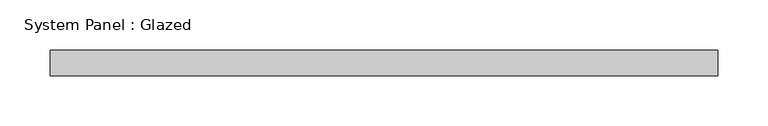
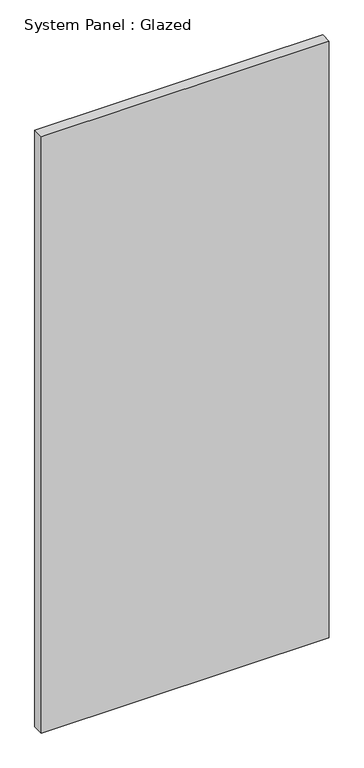
"""IFC4 building model written with IfcOpenShell, lengths in millimetres: plate geometry, System Panel : Glazed."""

from ifc_helpers import new_model, si_unit, origin, origin_with_axes, place, context, project, spatial, polyline, outline, extrude, source, transform, mapped, element, save


def system_panel_glazed_c34084c8(model_context):
    return source(origin(), model_context, "Body", "SweptSolid", [
        extrude(outline(polyline([(333.375, 19.05), (-333.375, 19.05), (-333.375, 44.45), (333.375, 44.45), (333.375, 19.05)])), origin_with_axes(), (0.0, 0.0, 1.0), 1459.1267095),
    ])


if __name__ == "__main__":
    model = new_model("IFC4")
    model_context = context("Model", 3, world=origin())
    ifc_project = project(units=[si_unit("LENGTHUNIT", "METRE", prefix="MILLI")], contexts=[model_context])
    site = spatial("IfcSite", under=ifc_project)
    building = spatial("IfcBuilding", under=site)
    placement = place(None, origin())
    system_panel_glazed_shape = system_panel_glazed_c34084c8(model_context)
    element("IfcPlate", 1, ObjectType="System Panel : Glazed", at=placement, inside=building, context=model_context, shape_type="MappedRepresentation", body=[
        mapped(system_panel_glazed_shape, transform((0.0, 0.0, 0.0), x_axis=(1.0, 0.0, 0.0), y_axis=(0.0, 1.0, 0.0), z_axis=(0.0, 0.0, 1.0))),
    ])
    save(model, "model.ifc")

# Revit data of these elements
# Type "System Panel : Glazed"
#   Construction Type Id = "GSP4R"
#   Analytic Construction = "1/8 in Pilkington single glazing"
#   Visual Light Transmittance = 0.9
#   Solar Heat Gain Coefficient = 0.86
#   Heat Transfer Coefficient (U) = 1.18115 BTU/(h·ft²·°F)
#   Define Thermal Properties by = 1
# Element 1 (IfcPlate, "System Panel : Glazed")
#   Materials on its faces: "Glass"
# Materials
#   "Glass": class "Glass", colour RGB 0 128 192, transparency 0.75, Description = "Soda Lime Glass", Cost = 0
